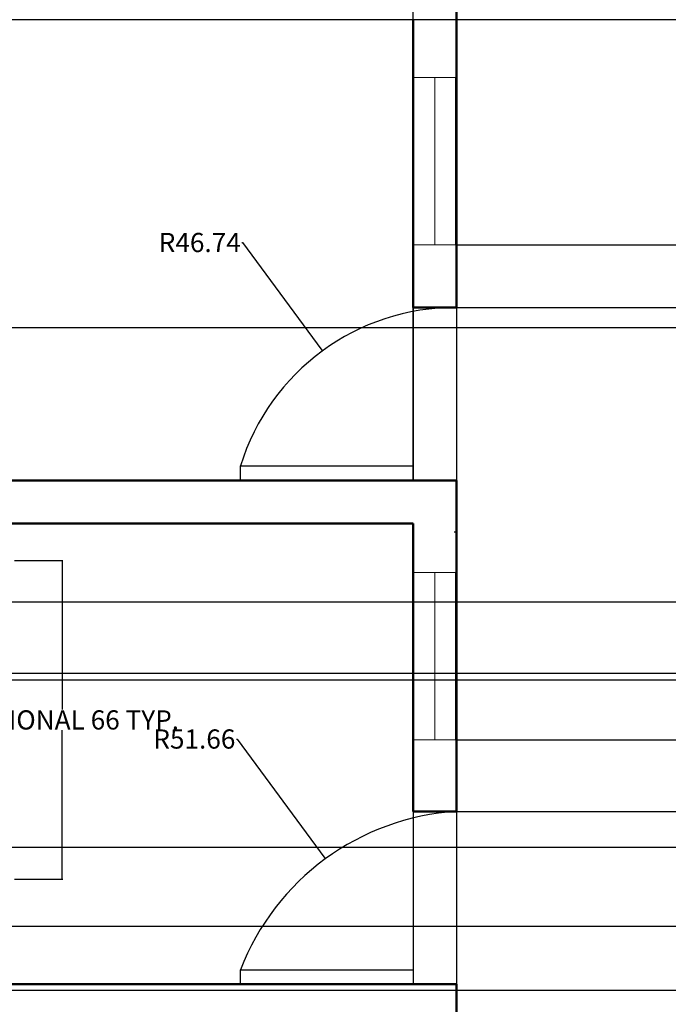
# Model space of a CAD drawing. Units: inches. Extents: x 1454 to 2136, y 626 to 1213.
# Tile 3 of 23: x 1564 to 1699, y 768 to 973. Entities that reach past the tile are written whole.
import ezdxf

# ---------------------------------------------------------------- set-up
doc = ezdxf.new("R2010")
doc.units = ezdxf.units.IN
doc.header["$MEASUREMENT"] = 0
for name, color, linetype, lineweight in [('A-ANNO-DIMS', 2, 'Continuous', 18), ('A-DOOR', 3, 'Continuous', 25), ('A-FURN-PATT', 252, 'Continuous', 13), ('A-GLAZ', 4, 'Continuous', 18), ('A-PLNT-PATT', 116, 'Continuous', 13), ('A-WALL', 7, 'Continuous', 50)]:
    doc.layers.add(name, color=color, linetype=linetype, lineweight=lineweight)
doc.styles.get("Standard").update_dxf_attribs({"font": 'arial.ttf'})
doc.dimstyles.get("Standard").update_dxf_attribs({"dimtxt": 4, "dimasz": 0.18, "dimexe": 0.18, "dimexo": 0.0625, "dimgap": 0.09, "dimtad": 0, "dimtih": 1, "dimtoh": 1, "dimdec": 0, "dimrnd": 6, "dimzin": 0, "dimdsep": 46, "dimlunit": 3, "dimtxsty": 'Standard', "dimcen": 0.09, "dimadec": 0, "dimazin": 0, "dimtfac": 1, "dimtdec": 0, "dimtofl": 0, "dimtmove": 0, "dimatfit": 3, "dimfxl": 1, "dimtolj": 1, "dimtzin": 0, "dimarcsym": 0})

# ---------------------------------------------------------------- blocks, each defined once
blk = doc.blocks.new('WIN-34_84')
blk.add_line((34.84, 4.31), (0, 4.31))
blk.add_lwpolyline([(34.84, 0), (0, 0), (0, 9), (34.84, 9)], close=True)
blk = doc.blocks.new('DOOR-LEAF-36')
blk.add_lwpolyline([(-36, 3), (0, 3), (0, 0), (-36, 0)], close=True)
blk = doc.blocks.new('*D13')
at = {"layer": 'A-ANNO-DIMS', "color": 0, "lineweight": -2, "transparency": 16777216}
for p, q in [((1562.49, 860.58), (1572.58, 860.58)), ((1572.4, 860.4), (1572.4, 829.52)), ((1572.4, 794.32), (1572.4, 825.2)), ((1562.49, 794.14), (1572.58, 794.14))]:
    blk.add_line(p, q, dxfattribs=at)
at = {"layer": 'A-ANNO-DIMS', "color": 0, "transparency": 16777216}
for points in [[(1572.37, 860.4), (1572.43, 860.4), (1572.4, 860.58)], [(1572.37, 794.32), (1572.43, 794.32), (1572.4, 794.14)]]:
    blk.add_solid(points, dxfattribs=at)
at = {"layer": 'Defpoints', "color": 0, "transparency": 16777216}
for p in [(1562.43, 860.58), (1562.43, 794.14), (1572.4, 794.14)]:
    blk.add_point(p, dxfattribs=at)
at = {"layer": 'A-ANNO-DIMS', "color": 0, "transparency": 16777216, "insert": (1572.4, 827.36), "char_height": 4, "attachment_point": 5}
blk.add_mtext('\\A1;SECTIONAL 66 TYP.', dxfattribs=at)
blk = doc.blocks.new('*D40')
at = {"layer": 'A-ANNO-DIMS', "color": 0, "lineweight": -2, "transparency": 16777216}
for p, q in [((1501.56, 877.34), (1501.56, 1210.46)), ((1501.74, 1210.28), (1569.24, 1210.28)), ((1645.38, 1210.28), (1577.87, 1210.28)), ((1645.56, 877.34), (1645.56, 1210.46))]:
    blk.add_line(p, q, dxfattribs=at)
at = {"layer": 'A-ANNO-DIMS', "color": 0, "transparency": 16777216}
for points in [[(1501.74, 1210.31), (1501.74, 1210.25), (1501.56, 1210.28)], [(1645.38, 1210.31), (1645.38, 1210.25), (1645.56, 1210.28)]]:
    blk.add_solid(points, dxfattribs=at)
at = {"layer": 'Defpoints', "color": 0, "transparency": 16777216}
for p in [(1645.56, 1210.28), (1501.56, 877.28), (1645.56, 877.28)]:
    blk.add_point(p, dxfattribs=at)
at = {"layer": 'A-ANNO-DIMS', "color": 0, "transparency": 16777216, "insert": (1573.56, 1210.28), "char_height": 4, "attachment_point": 5}
blk.add_mtext('\\A1;144', dxfattribs=at)
blk = doc.blocks.new('*D41')
at = {"layer": 'A-ANNO-DIMS', "color": 0, "lineweight": -2, "transparency": 16777216}
for p, q in [((1645.49, 772.28), (1462.37, 772.28)), ((1462.55, 772.1), (1462.55, 721.91)), ((1462.55, 667.46), (1462.55, 717.65)), ((1645.49, 667.28), (1462.37, 667.28))]:
    blk.add_line(p, q, dxfattribs=at)
at = {"layer": 'A-ANNO-DIMS', "color": 0, "transparency": 16777216}
for points in [[(1462.52, 772.1), (1462.58, 772.1), (1462.55, 772.28)], [(1462.52, 667.46), (1462.58, 667.46), (1462.55, 667.28)]]:
    blk.add_solid(points, dxfattribs=at)
at = {"layer": 'Defpoints', "color": 0, "transparency": 16777216}
for p in [(1462.55, 772.28), (1645.56, 772.28), (1645.56, 667.28)]:
    blk.add_point(p, dxfattribs=at)
at = {"layer": 'A-ANNO-DIMS', "color": 0, "transparency": 16777216, "insert": (1462.55, 719.78), "char_height": 4, "attachment_point": 5}
blk.add_mtext('\\A1;105', dxfattribs=at)
blk = doc.blocks.new('*D42')
at = {"layer": 'A-ANNO-DIMS', "color": 0, "lineweight": -2, "transparency": 16777216}
for p, q in [((1645.49, 877.28), (1462.37, 877.28)), ((1462.55, 877.1), (1462.55, 826.91)), ((1462.55, 772.46), (1462.55, 822.65)), ((1645.49, 772.28), (1462.37, 772.28))]:
    blk.add_line(p, q, dxfattribs=at)
at = {"layer": 'A-ANNO-DIMS', "color": 0, "transparency": 16777216}
for points in [[(1462.52, 877.1), (1462.58, 877.1), (1462.55, 877.28)], [(1462.52, 772.46), (1462.58, 772.46), (1462.55, 772.28)]]:
    blk.add_solid(points, dxfattribs=at)
at = {"layer": 'Defpoints', "color": 0, "transparency": 16777216}
for p in [(1462.55, 877.28), (1645.56, 877.28), (1645.56, 772.28)]:
    blk.add_point(p, dxfattribs=at)
at = {"layer": 'A-ANNO-DIMS', "color": 0, "transparency": 16777216, "insert": (1462.55, 824.78), "char_height": 4, "attachment_point": 5}
blk.add_mtext('\\A1;105', dxfattribs=at)
blk = doc.blocks.new('*D45')
at = {"layer": 'A-ANNO-DIMS', "color": 0, "lineweight": -2, "transparency": 16777216}
for p, q in [((1654.56, 913.34), (1654.56, 1210.46)), ((1654.74, 1210.28), (1670.92, 1210.28)), ((1700.9, 1210.28), (1684.72, 1210.28)), ((1701.08, 909.11), (1701.08, 1210.46))]:
    blk.add_line(p, q, dxfattribs=at)
at = {"layer": 'A-ANNO-DIMS', "color": 0, "transparency": 16777216}
for points in [[(1654.74, 1210.31), (1654.74, 1210.25), (1654.56, 1210.28)], [(1700.9, 1210.31), (1700.9, 1210.25), (1701.08, 1210.28)]]:
    blk.add_solid(points, dxfattribs=at)
at = {"layer": 'Defpoints', "color": 0, "transparency": 16777216}
for p in [(1701.08, 1210.28), (1654.56, 913.28), (1701.08, 909.05)]:
    blk.add_point(p, dxfattribs=at)
at = {"layer": 'A-ANNO-DIMS', "color": 0, "transparency": 16777216, "insert": (1677.82, 1210.28), "char_height": 4, "attachment_point": 5}
blk.add_mtext('\\A1;46.52', dxfattribs=at)
blk = doc.blocks.new('*D46')
at = {"layer": 'A-ANNO-DIMS', "color": 0, "lineweight": -2, "transparency": 16777216}
for p, q in [((1701.01, 909.05), (1462.37, 909.05)), ((1462.55, 908.87), (1462.55, 842.13)), ((1462.55, 771.13), (1462.55, 837.86)), ((1753.01, 770.95), (1462.37, 770.95))]:
    blk.add_line(p, q, dxfattribs=at)
at = {"layer": 'A-ANNO-DIMS', "color": 0, "transparency": 16777216}
for points in [[(1462.52, 908.87), (1462.58, 908.87), (1462.55, 909.05)], [(1462.52, 771.13), (1462.58, 771.13), (1462.55, 770.95)]]:
    blk.add_solid(points, dxfattribs=at)
at = {"layer": 'Defpoints', "color": 0, "transparency": 16777216}
for p in [(1701.08, 909.05), (1462.55, 770.95), (1753.08, 770.95)]:
    blk.add_point(p, dxfattribs=at)
at = {"layer": 'A-ANNO-DIMS', "color": 0, "transparency": 16777216, "insert": (1462.55, 840), "char_height": 4, "attachment_point": 5}
blk.add_mtext('\\A1;138.1', dxfattribs=at)
blk = doc.blocks.new('*D48')
at = {"layer": 'A-ANNO-DIMS', "color": 0, "lineweight": -2, "transparency": 16777216}
for p, q in [((1879.49, 973.28), (1462.37, 973.28)), ((1462.55, 973.1), (1462.55, 943.3)), ((1462.55, 909.23), (1462.55, 939.03)), ((1885.19, 909.05), (1462.37, 909.05))]:
    blk.add_line(p, q, dxfattribs=at)
at = {"layer": 'A-ANNO-DIMS', "color": 0, "transparency": 16777216}
for points in [[(1462.52, 973.1), (1462.58, 973.1), (1462.55, 973.28)], [(1462.52, 909.23), (1462.58, 909.23), (1462.55, 909.05)]]:
    blk.add_solid(points, dxfattribs=at)
at = {"layer": 'Defpoints', "color": 0, "transparency": 16777216}
for p in [(1879.56, 973.28), (1462.55, 909.05), (1885.25, 909.05)]:
    blk.add_point(p, dxfattribs=at)
at = {"layer": 'A-ANNO-DIMS', "color": 0, "transparency": 16777216, "insert": (1462.55, 941.17), "char_height": 4, "attachment_point": 5}
blk.add_mtext('\\A1;64.23', dxfattribs=at)
blk = doc.blocks.new('*D52')
at = {"layer": 'A-ANNO-DIMS', "color": 0, "lineweight": -2, "transparency": 16777216}
for p, q in [((1927.57, 800.77), (1462.37, 800.77)), ((1462.55, 800.59), (1462.55, 794.66)), ((1462.55, 784.46), (1462.55, 790.4)), ((1927.49, 784.28), (1462.37, 784.28))]:
    blk.add_line(p, q, dxfattribs=at)
at = {"layer": 'A-ANNO-DIMS', "color": 0, "transparency": 16777216}
for points in [[(1462.52, 800.59), (1462.58, 800.59), (1462.55, 800.77)], [(1462.52, 784.46), (1462.58, 784.46), (1462.55, 784.28)]]:
    blk.add_solid(points, dxfattribs=at)
at = {"layer": 'Defpoints', "color": 0, "transparency": 16777216}
for p in [(1462.55, 800.77), (1927.64, 800.77), (1927.56, 784.28)]:
    blk.add_point(p, dxfattribs=at)
at = {"layer": 'A-ANNO-DIMS', "color": 0, "transparency": 16777216, "insert": (1462.55, 792.53), "char_height": 4, "attachment_point": 5}
blk.add_mtext('\\A1;16.49', dxfattribs=at)
blk = doc.blocks.new('*D53')
at = {"layer": 'A-ANNO-DIMS', "color": 0, "lineweight": -2, "transparency": 16777216}
for p, q in [((1927.57, 851.9), (1462.37, 851.9)), ((1462.55, 851.72), (1462.55, 845.89)), ((1462.55, 835.79), (1462.55, 841.63)), ((1927.57, 835.61), (1462.37, 835.61))]:
    blk.add_line(p, q, dxfattribs=at)
at = {"layer": 'A-ANNO-DIMS', "color": 0, "transparency": 16777216}
for points in [[(1462.52, 851.72), (1462.58, 851.72), (1462.55, 851.9)], [(1462.52, 835.79), (1462.58, 835.79), (1462.55, 835.61)]]:
    blk.add_solid(points, dxfattribs=at)
at = {"layer": 'Defpoints', "color": 0, "transparency": 16777216}
for p in [(1462.55, 851.9), (1927.64, 851.9), (1927.64, 835.61)]:
    blk.add_point(p, dxfattribs=at)
at = {"layer": 'A-ANNO-DIMS', "color": 0, "transparency": 16777216, "insert": (1462.55, 843.76), "char_height": 4, "attachment_point": 5}
blk.add_mtext('\\A1;16.29', dxfattribs=at)
blk = doc.blocks.new('*D57')
at = {"layer": 'A-ANNO-DIMS', "color": 0, "lineweight": -2, "transparency": 16777216}
for p, q in [((1654.43, 823.23), (2122.74, 823.23)), ((2122.56, 823.05), (2122.56, 817.89)), ((2122.56, 808.46), (2122.56, 813.62)), ((1654.62, 808.28), (2122.74, 808.28))]:
    blk.add_line(p, q, dxfattribs=at)
at = {"layer": 'A-ANNO-DIMS', "color": 0, "transparency": 16777216}
for points in [[(2122.53, 823.05), (2122.59, 823.05), (2122.56, 823.23)], [(2122.53, 808.46), (2122.59, 808.46), (2122.56, 808.28)]]:
    blk.add_solid(points, dxfattribs=at)
at = {"layer": 'Defpoints', "color": 0, "transparency": 16777216}
for p in [(1654.37, 823.23), (2122.56, 823.23), (1654.56, 808.28)]:
    blk.add_point(p, dxfattribs=at)
at = {"layer": 'A-ANNO-DIMS', "color": 0, "transparency": 16777216, "insert": (2122.56, 815.75), "char_height": 4, "attachment_point": 5}
blk.add_mtext('\\A1;14.944', dxfattribs=at)
blk = doc.blocks.new('*D58')
at = {"layer": 'A-ANNO-DIMS', "color": 0, "lineweight": -2, "transparency": 16777216}
for p, q in [((1654.43, 926.36), (2122.74, 926.36)), ((2122.56, 926.18), (2122.56, 921.96)), ((2122.56, 913.46), (2122.56, 917.69)), ((1654.62, 913.28), (2122.74, 913.28))]:
    blk.add_line(p, q, dxfattribs=at)
at = {"layer": 'A-ANNO-DIMS', "color": 0, "transparency": 16777216}
for points in [[(2122.53, 926.18), (2122.59, 926.18), (2122.56, 926.36)], [(2122.53, 913.46), (2122.59, 913.46), (2122.56, 913.28)]]:
    blk.add_solid(points, dxfattribs=at)
at = {"layer": 'Defpoints', "color": 0, "transparency": 16777216}
for p in [(1654.37, 926.36), (2122.56, 926.36), (1654.56, 913.28)]:
    blk.add_point(p, dxfattribs=at)
at = {"layer": 'A-ANNO-DIMS', "color": 0, "transparency": 16777216, "insert": (2122.56, 919.82), "char_height": 4, "attachment_point": 5}
blk.add_mtext('\\A1;13.082', dxfattribs=at)
blk = doc.blocks.new('*D65')
at = {"layer": 'A-ANNO-DIMS', "color": 0, "lineweight": -2, "transparency": 16777216}
for p, q in [((1885.19, 909.05), (1462.37, 909.05)), ((1462.55, 908.87), (1462.55, 875.15)), ((1462.55, 837.23), (1462.55, 870.95)), ((1885.19, 837.05), (1462.37, 837.05))]:
    blk.add_line(p, q, dxfattribs=at)
at = {"layer": 'A-ANNO-DIMS', "color": 0, "transparency": 16777216}
for points in [[(1462.52, 908.87), (1462.58, 908.87), (1462.55, 909.05)], [(1462.52, 837.23), (1462.58, 837.23), (1462.55, 837.05)]]:
    blk.add_solid(points, dxfattribs=at)
at = {"layer": 'Defpoints', "color": 0, "transparency": 16777216}
for p in [(1885.25, 909.05), (1462.55, 837.05), (1885.25, 837.05)]:
    blk.add_point(p, dxfattribs=at)
at = {"layer": 'A-ANNO-DIMS', "color": 0, "transparency": 16777216, "insert": (1462.55, 873.05), "char_height": 4, "attachment_point": 5}
blk.add_mtext('\\A1;72', dxfattribs=at)
blk = doc.blocks.new('*D91')
at = {"layer": 'A-ANNO-DIMS', "color": 0, "lineweight": -2, "transparency": 16777216}
for p, q in [((1608.71, 823.38), (1608.89, 823.38)), ((1608.89, 823.38), (1627.11, 798.53)), ((1657.68, 756.72), (1657.86, 756.72)), ((1657.77, 756.63), (1657.77, 756.81))]:
    blk.add_line(p, q, dxfattribs=at)
at = {"layer": 'A-ANNO-DIMS', "color": 0, "transparency": 16777216}
blk.add_solid([(1627.13, 798.54), (1627.09, 798.51), (1627.22, 798.38)], dxfattribs=at)
at = {"layer": 'Defpoints', "color": 0, "transparency": 16777216}
for p in [(1627.22, 798.38), (1657.77, 756.72)]:
    blk.add_point(p, dxfattribs=at)
at = {"layer": 'A-ANNO-DIMS', "color": 0, "transparency": 16777216, "insert": (1599.95, 823.38), "char_height": 4, "attachment_point": 5}
blk.add_mtext('\\A1;R51.66', dxfattribs=at)
blk = doc.blocks.new('*D92')
at = {"layer": 'A-ANNO-DIMS', "color": 0, "lineweight": -2, "transparency": 16777216}
for p, q in [((1608.77, 1030.83), (1608.95, 1030.83)), ((1608.86, 1030.74), (1608.86, 1030.92)), ((1554.95, 972.02), (1575.05, 993.94)), ((1554.77, 972.02), (1554.95, 972.02))]:
    blk.add_line(p, q, dxfattribs=at)
at = {"layer": 'A-ANNO-DIMS', "color": 0, "transparency": 16777216}
blk.add_solid([(1575.02, 993.96), (1575.07, 993.92), (1575.17, 994.07)], dxfattribs=at)
at = {"layer": 'Defpoints', "color": 0, "transparency": 16777216}
for p in [(1608.86, 1030.83), (1575.17, 994.07)]:
    blk.add_point(p, dxfattribs=at)
at = {"layer": 'A-ANNO-DIMS', "color": 0, "transparency": 16777216, "insert": (1546.02, 972.02), "char_height": 4, "attachment_point": 5}
blk.add_mtext('\\A1;R49.86', dxfattribs=at)
blk = doc.blocks.new('*D93')
at = {"layer": 'A-ANNO-DIMS', "color": 0, "lineweight": -2, "transparency": 16777216}
for p, q in [((1609.83, 926.85), (1610.01, 926.85)), ((1610.01, 926.85), (1626.48, 904.38)), ((1654.14, 866.54), (1654.32, 866.54)), ((1654.23, 866.45), (1654.23, 866.63))]:
    blk.add_line(p, q, dxfattribs=at)
at = {"layer": 'A-ANNO-DIMS', "color": 0, "transparency": 16777216}
blk.add_solid([(1626.51, 904.4), (1626.46, 904.36), (1626.59, 904.23)], dxfattribs=at)
at = {"layer": 'Defpoints', "color": 0, "transparency": 16777216}
for p in [(1626.59, 904.23), (1654.23, 866.54)]:
    blk.add_point(p, dxfattribs=at)
at = {"layer": 'A-ANNO-DIMS', "color": 0, "transparency": 16777216, "insert": (1601.08, 926.85), "char_height": 4, "attachment_point": 5}
blk.add_mtext('\\A1;R46.74', dxfattribs=at)

msp = doc.modelspace()

# ---------------------------------------------------------------- hatches: boundary and pattern name
at = {"layer": 'A-FURN-PATT'}
h = msp.add_hatch(dxfattribs=at)
h.set_pattern_fill('ESCHER', color=256)
h.paths.add_polyline_path([(1511.3761, 923.7174, 1), (1525.379, 923.7174, 1)])
h.paths.add_polyline_path([(1525.379, 816.0542, 1), (1511.3761, 816.0542, 1)])
h.paths.add_polyline_path([(1525.379, 712.7345, 1), (1511.3761, 712.7345, 1)])
h.paths.add_polyline_path([(2070.5057, 794.3402, 1), (2056.5027, 794.3402, 1)])
h.paths.add_polyline_path([(2005.868, 1014.5578, 1), (1991.8651, 1014.5578, 1)])
h.paths.add_polyline_path([(1994.0647, 1066.7584, 1), (2008.0677, 1066.7584, 1)])
h.paths.add_polyline_path([(1919.5492, 1065.3848, 1), (1933.5521, 1065.3848, 1)])
h.paths.add_polyline_path([(1936.8517, 1013.7336, 1), (1922.8488, 1013.7336, 1)])
h.paths.add_polyline_path([(1824.6062, 1109.1557, 1), (1838.6091, 1109.1557, 1)])
at = {"layer": 'A-PLNT-PATT'}
h = msp.add_hatch(dxfattribs=at)
h.set_pattern_fill('ESCHER', color=256)
h.paths.add_polyline_path([(1767.2815, 694.0009, 1), (1753.2786, 694.0009, 1)])
h.paths.add_polyline_path([(1578.6873, 1043.8029, 1), (1564.6844, 1043.8029, 1)])

# ---------------------------------------------------------------- linework, layer by layer
at = {"layer": 'A-DOOR'}
for p, q in [((1645.5563, 913.2825), (1645.5563, 877.2825)), ((1654.5563, 913.2825), (1654.5563, 877.2825)), ((1645.5563, 808.2825), (1645.5563, 772.2825)), ((1654.5563, 808.2825), (1654.5563, 772.2825))]:
    msp.add_line(p, q, dxfattribs=at)
for centre, radius, start, end in [((1654.2317, 866.5433), 46.7403, 89.602076, 162.905599), ((1657.7683, 756.7207), 51.6617, 93.564522, 158.943153)]:
    msp.add_arc(centre, radius, start, end, dxfattribs=at)
at = {"layer": 'A-WALL'}
for p, q in [((1654.5563, 982.2825), (1654.5563, 913.2825)), ((1645.5563, 973.2825), (1645.5563, 913.2825)), ((1654.5563, 913.2825), (1645.5563, 913.2825)), ((1654.5563, 877.2825), (1501.5563, 877.2825)), ((1654.5563, 877.2825), (1654.5563, 808.2825)), ((1645.5563, 868.2825), (1501.5563, 868.2825)), ((1645.5563, 868.2825), (1645.5563, 808.2825)), ((1654.5563, 808.2825), (1645.5563, 808.2825)), ((1654.5563, 772.2825), (1501.5563, 772.2825)), ((1654.5563, 772.2825), (1654.5563, 703.2825))]:
    msp.add_line(p, q, dxfattribs=at)

# ---------------------------------------------------------------- block references
at = {"layer": 'A-DOOR'}
for p in [(1645.5563, 877.2825), (1645.5563, 772.2825)]:
    msp.add_blockref('DOOR-LEAF-36', p, dxfattribs=at)
at = {"layer": 'A-GLAZ'}
for p, rotation in [((1654.3723, 926.364), 89.99999999999984), ((1654.3723, 823.2266), 89.99999999999991)]:
    msp.add_blockref('WIN-34_84', p, dxfattribs=dict(at, rotation=rotation))

# ---------------------------------------------------------------- dimensions: what is measured, and where the dimension line sits
at = {"layer": 'A-ANNO-DIMS'}
for base, p1, p2, override, picture, middle in [((1645.5563, 1210.2845), (1501.5563, 877.2825), (1645.5563, 877.2825), {"dimdec": 0, "dimlfac": 1, "dimrnd": 0, "dimzin": 0, "dimdsep": 46, "dimlunit": 2}, '*D40', (1573.5563, 1210.2845)), ((1701.0763, 1210.2845), (1654.5563, 913.2825), (1701.0763, 909.0476), {"dimdec": 2, "dimlfac": 1, "dimrnd": 0, "dimzin": 0, "dimdsep": 46, "dimlunit": 2}, '*D45', (1677.8163, 1210.2845))]:
    dim = msp.add_linear_dim(base=base, p1=p1, p2=p2, dimstyle='Standard', override=override, dxfattribs=at)
    dim.commit()
    dim.dimension.update_dxf_attribs({"geometry": picture, "text_midpoint": middle})
for center, mpoint, picture, middle in [((1608.86, 1030.8286), (1575.1679, 994.0729), '*D92', (1546.0211, 972.0196)), ((1654.2317, 866.5433), (1626.5911, 904.2348), '*D93', (1601.0819, 926.8498)), ((1657.7683, 756.7207), (1627.2172, 798.3808), '*D91', (1599.9548, 823.3768))]:
    dim = msp.add_radius_dim(center=center, mpoint=mpoint, dimstyle='Standard', override={"dimdec": 2, "dimlfac": 1, "dimrnd": 0, "dimzin": 0, "dimdsep": 46, "dimlunit": 2}, dxfattribs=at)
    dim.commit()
    dim.dimension.update_dxf_attribs({"geometry": picture, "text_midpoint": middle, "dimtype": 164})
for base, p1, p2, override, picture, middle in [((1462.5543, 909.0476), (1879.5563, 973.2825), (1885.2497, 909.0476), {"dimdec": 2, "dimlfac": 1, "dimrnd": 0, "dimzin": 0, "dimdsep": 46, "dimlunit": 2}, '*D48', (1462.5543, 941.165)), ((2122.55832, 926.36405), (1654.55632, 913.28246), (1654.37233, 926.36405), {"dimdec": 3, "dimlfac": 1, "dimrnd": 0, "dimzin": 0, "dimdsep": 46, "dimlunit": 2}, '*D58', (2122.55832, 919.82325)), ((1462.5543, 770.9473), (1701.0763, 909.0476), (1753.0763, 770.9473), {"dimdec": 1, "dimlfac": 1, "dimrnd": 0, "dimzin": 0, "dimdsep": 46, "dimlunit": 2}, '*D46', (1462.5543, 839.9975)), ((1462.5543, 837.0476), (1885.2497, 909.0476), (1885.2497, 837.0476), {"dimdec": 0, "dimlfac": 1, "dimrnd": 0, "dimzin": 0, "dimdsep": 46, "dimlunit": 2}, '*D65', (1462.5543, 873.0476)), ((1462.5543, 877.2825), (1645.5563, 772.2825), (1645.5563, 877.2825), {"dimdec": 0, "dimlfac": 1, "dimrnd": 0, "dimzin": 0, "dimdsep": 46, "dimlunit": 2}, '*D42', (1462.5543, 824.7825)), ((1462.5543, 851.9027), (1927.6352, 835.6136), (1927.6352, 851.9027), {"dimdec": 2, "dimlfac": 1, "dimrnd": 0, "dimzin": 0, "dimdsep": 46, "dimlunit": 2}, '*D53', (1462.5543, 843.7581)), ((2122.5583, 823.2266), (1654.5563, 808.2825), (1654.3723, 823.2266), {"dimdec": 3, "dimlfac": 1, "dimrnd": 0, "dimzin": 0, "dimdsep": 46, "dimlunit": 2}, '*D57', (2122.5583, 815.7545)), ((1462.5543, 800.7734), (1927.5563, 784.2825), (1927.6352, 800.7734), {"dimdec": 2, "dimlfac": 1, "dimrnd": 0, "dimzin": 0, "dimdsep": 46, "dimlunit": 2}, '*D52', (1462.5543, 792.5279)), ((1462.5543, 772.2825), (1645.5563, 667.2825), (1645.5563, 772.2825), {"dimdec": 0, "dimlfac": 1, "dimrnd": 0, "dimzin": 0, "dimdsep": 46, "dimlunit": 2}, '*D41', (1462.5543, 719.7825))]:
    dim = msp.add_linear_dim(base=base, p1=p1, p2=p2, angle=90, dimstyle='Standard', override=override, dxfattribs=at)
    dim.commit()
    dim.dimension.update_dxf_attribs({"geometry": picture, "text_midpoint": middle})
dim = msp.add_linear_dim(base=(1572.3962, 794.1444), p1=(1562.4308, 860.5807), p2=(1562.4308, 794.1444), angle=270, text='SECTIONAL <> TYP.', dimstyle='Standard', override={"dimdec": 0, "dimlfac": 1, "dimrnd": 0, "dimzin": 0, "dimdsep": 46, "dimlunit": 2}, dxfattribs=at)
dim.commit()
dim.dimension.update_dxf_attribs({"geometry": '*D13', "text_midpoint": (1572.3962, 827.3626)})

doc.saveas('drawing.dxf')
